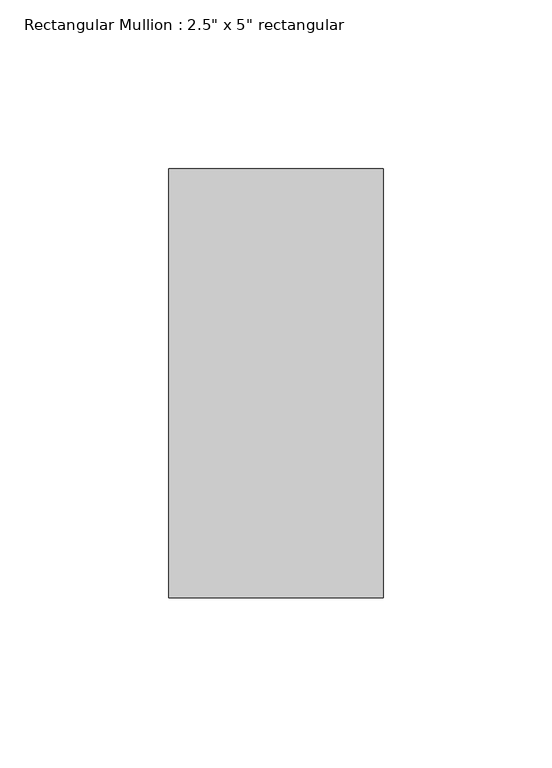
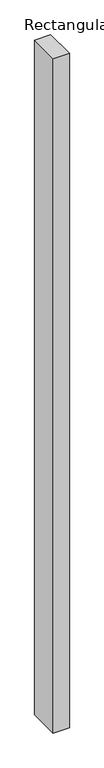
"""IFC4 building model written with IfcOpenShell, lengths in millimetres: member geometry."""

from ifc_helpers import new_model, si_unit, frame, origin, place, context, project, spatial, polyline, outline, extrude, source, transform, mapped, element, save


def member_1b94d493(model_context):
    return source(origin(), model_context, "Body", "SweptSolid", [
        extrude(outline(polyline([(0.0, 63.5), (0.0, -63.5), (-63.5, -63.5), (-63.5, 63.5), (0.0, 63.5)])), frame((0.0, 0.0, -2816.4340209), z_axis=(0.0, 0.0, 1.0), x_axis=(1.0, 0.0, 0.0)), (0.0, 0.0, 1.0), 2816.4340209),
    ])


if __name__ == "__main__":
    model = new_model("IFC4")
    model_context = context("Model", 3, world=origin())
    ifc_project = project(units=[si_unit("LENGTHUNIT", "METRE", prefix="MILLI")], contexts=[model_context])
    site = spatial("IfcSite", under=ifc_project)
    building = spatial("IfcBuilding", under=site)
    placement = place(None, origin())
    member_shape = member_1b94d493(model_context)
    element("IfcMember", 1, ObjectType="Rectangular Mullion : 2.5\" x 5\" rectangular", at=placement, inside=building, context=model_context, shape_type="MappedRepresentation", body=[
        mapped(member_shape, transform((0.0, 0.0, 0.0), x_axis=(1.0, 0.0, 0.0), y_axis=(0.0, 1.0, 0.0), z_axis=(0.0, 0.0, 1.0))),
    ])
    save(model, "model.ifc")

# Revit data of these elements
# Type "Rectangular Mullion : 2.5\" x 5\" rectangular"
#   built-in parameter 1007304 = 0.416667 (stored number, unit not read)
#   built-in parameter 1007301 = 0.104167 (stored number, unit not read)
#   built-in parameter 1007300 = 0.104167 (stored number, unit not read)
# Element 1 (IfcMember, "Rectangular Mullion : 2.5\" x 5\" rectangular")
#   Materials on its faces: "Aluminum"
# Materials
#   "Aluminum": class "Metal", colour RGB 247 247 247, transparency 0, Description = "Aluminum 6061", Cost = 0
